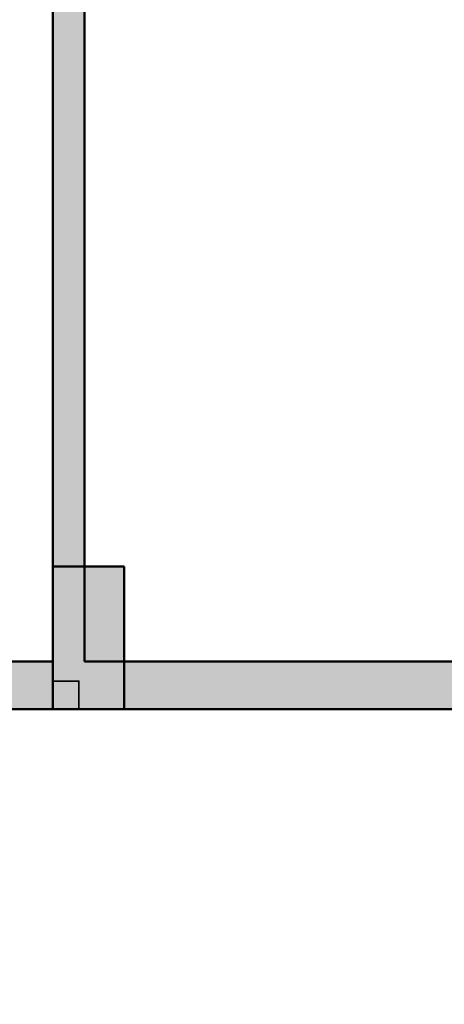
# Model space of a CAD drawing. Units: inches. Extents: x -7 to 1228, y -146 to 1091.
# Tile 58 of 88: x 376 to 429, y 531 to 655. Entities that reach past the tile are written whole.
import ezdxf

# ---------------------------------------------------------------- set-up
doc = ezdxf.new("R2010")
doc.units = ezdxf.units.IN
for name, color, linetype, lineweight in [('A-COLS', 6, 'Continuous', 35), ('A-WALL', 7, 'Continuous', 50), ('A-WALL-PATT', 251, 'Continuous', 13)]:
    doc.layers.add(name, color=color, linetype=linetype, lineweight=lineweight)

msp = doc.modelspace()

# ---------------------------------------------------------------- hatches: boundary and pattern name
at = {"layer": 'A-COLS'}
h = msp.add_hatch(color=256, dxfattribs=at)
h.dxf.hatch_style = 1
h.paths.add_polyline_path([(389, 586), (380, 586), (380, 571.55), (383.29, 571.55), (383.29, 568), (389, 568)])
h = msp.add_hatch(color=256, dxfattribs=at)
h.dxf.hatch_style = 1
h.paths.add_polyline_path([(383.29, 571.55), (380, 571.55), (380, 568), (383.29, 568)])
at = {"layer": 'A-WALL-PATT'}
h = msp.add_hatch(color=256, dxfattribs=at)
h.dxf.hatch_style = 1
h.paths.add_polyline_path([(69, 568), (60, 568), (60, 493), (63.29, 493), (69, 493)])
h.paths.add_polyline_path([(69, 662.41), (60, 662.41), (60, 586), (69, 586)], flags=17)
h.paths.add_polyline_path([(69, 723), (184, 723), (184, 734), (179, 734), (179, 728), (69, 728), (69, 741.62), (60, 741.62), (60, 698.41), (69, 698.41)], flags=17)
h.paths.add_polyline_path([(69, 782), (231, 782), (231, 728), (231, 723), (231, 586), (236, 586), (236, 787), (69, 787), (69, 800.13), (60, 800.13), (60, 765.62), (69, 765.62)])
h.paths.add_polyline_path([(184, 842), (189, 842), (189, 848), (173, 848), (173, 842), (179, 842), (179, 787), (184, 787)])
h.paths.add_polyline_path([(118.22, 69), (69, 69), (69, 60), (118.22, 60)])
h.paths.add_polyline_path([(227, 69), (154.22, 69), (154.22, 60), (227, 60)])
h.paths.add_polyline_path([(236, 60), (232.71, 60), (227, 60), (227, 36), (236, 36)])
h.paths.add_polyline_path([(389, 60), (380, 60), (380, 36), (389, 36)])
h.paths.add_polyline_path([(384, 181), (380, 181), (380, 115), (380, 78), (384, 78)])
h.paths.add_polyline_path([(380, 115), (334.55, 115), (334.55, 109), (380, 109)])
h.paths.add_polyline_path([(274.55, 115), (236, 115), (236, 201), (232.71, 201), (231, 201), (231, 78), (236, 78), (236, 109), (274.55, 109)])
h.paths.add_polyline_path([(69, 123), (60, 123), (60, 78), (69, 78)])
h.paths.add_polyline_path([(69, 201), (60, 201), (60, 159), (69, 159)])
h.paths.add_polyline_path([(143, 219), (69, 219), (69, 213), (143, 213)], flags=17)
h.paths.add_polyline_path([(189, 219), (184, 219), (184, 274), (231, 274), (231, 219), (236, 219), (236, 279), (184, 279), (184, 297), (179, 297), (179, 279), (69, 279), (69, 290.91), (60, 290.91), (60, 262.18), (69, 262.18), (69, 274), (179, 274), (179, 219), (173, 219), (173, 213), (189, 213)])
h.paths.add_polyline_path([(69, 238.18), (60, 238.18), (60, 219), (69, 219)], flags=17)
h.paths.add_polyline_path([(69, 333), (60, 333), (60, 314.91), (69, 314.91), (69, 316.96)])
h.paths.add_polyline_path([(190, 338), (184, 338), (69, 338), (69, 333), (179, 333), (179, 327), (184, 327), (184, 333.02), (190, 333.05)])
h.paths.add_polyline_path([(69, 386.81), (60, 386.81), (60, 351), (69, 351)])
h.paths.add_polyline_path([(69, 475), (60, 475), (60, 422.81), (69, 422.81)])
h.paths.add_polyline_path([(236, 475), (231, 475), (231, 351.24), (236, 351.24)])
h.paths.add_polyline_path([(384, 475), (380, 475), (380, 362), (384, 362)])
h.paths.add_polyline_path([(547, 307), (439, 307), (439, 356), (445, 356), (445, 362), (433, 362), (433, 307), (380, 307), (380, 244), (380, 241), (384, 241), (384, 301), (433, 301), (433, 277), (439, 277), (439, 301), (547, 301)])
h.paths.add_polyline_path([(547, 241), (439, 241), (439, 247), (433, 247), (433, 235), (547, 235)])
h.paths.add_polyline_path([(450, 69), (440.29, 69), (424.89, 69), (389, 69), (389, 60), (450, 60)])
h.paths.add_polyline_path([(547, 69), (486, 69), (486, 60), (547, 60)])
h.paths.add_polyline_path([(556, 148.27), (547, 148.27), (547, 78), (556, 78)])
h.paths.add_polyline_path([(556, 223), (547, 223), (547, 195), (547, 184.27), (556, 184.27)])
h.paths.add_polyline_path([(556, 311.19), (547, 311.19), (547, 273.08), (556, 273.08)])
h.paths.add_polyline_path([(556, 344), (552.71, 344), (547, 344), (547, 335.19), (556, 335.19)])
h.paths.add_polyline_path([(556, 249.08), (547, 249.08), (547, 241), (556, 241)])
h.paths.add_polyline_path([(547, 362), (475, 362), (475, 356), (547, 356)], flags=0)
h.paths.add_polyline_path([(556, 399.62), (547, 399.62), (547, 362), (556, 362)])
h.paths.add_polyline_path([(556, 475), (547, 475), (547, 435.62), (556, 435.62)])
h.paths.add_polyline_path([(547, 493), (389, 493), (389, 487), (547, 487)])
h.paths.add_polyline_path([(380, 493), (278, 493), (278, 487), (380, 487)])
h.paths.add_polyline_path([(227, 493), (69, 493), (69, 487), (227, 487)])
h.paths.add_polyline_path([(643, 122.44), (634, 122.44), (634, 78), (643, 78)])
h.paths.add_polyline_path([(702.5, 69), (692.79, 69), (677.39, 69), (643, 69), (643, 60), (702.5, 60)])
h.paths.add_polyline_path([(798, 69), (738.5, 69), (738.5, 60), (798, 60)])
h.paths.add_polyline_path([(807, 60), (803.71, 60), (798, 60), (798, 36), (807, 36)])
h.paths.add_polyline_path([(807, 109), (846.75, 109), (846.75, 115), (807, 115), (807, 159), (802, 159), (802, 78), (807, 78)])
h.paths.add_polyline_path([(807, 201), (802, 201), (802, 195), (807, 195)])
h.paths.add_polyline_path([(643, 201), (634, 201), (634, 158.44), (643, 158.44)])
h.paths.add_polyline_path([(756, 225), (751, 225), (751, 219), (643, 219), (643, 213), (756, 213)])
h.paths.add_polyline_path([(643, 240.85), (634, 240.85), (634, 219), (643, 219)])
h.paths.add_polyline_path([(643, 274), (643, 288.63), (634, 288.63), (634, 264.85), (643, 264.85)])
h.paths.add_polyline_path([(802, 279), (756, 279), (756, 297), (751, 297), (751, 279), (643, 279), (643, 274), (751, 274), (751, 255), (756, 255), (756, 274), (802, 274)])
h.paths.add_polyline_path([(807, 333), (803.71, 333), (802, 333), (802, 279), (802, 274), (802, 219), (807, 219)])
h.paths.add_polyline_path([(956, 182), (951, 182), (951, 115), (906.75, 115), (906.75, 109), (951, 109), (951, 78), (956, 78)])
h.paths.add_polyline_path([(960, 60), (951, 60), (951, 36), (960, 36)])
h.paths.add_polyline_path([(1021, 69), (1005.78, 69), (960, 69), (960, 60), (1021, 60)])
h.paths.add_polyline_path([(956, 224), (951, 224), (951, 218), (956, 218)])
h.paths.add_polyline_path([(956, 302), (1004, 302), (1004, 278), (1010, 278), (1010, 302), (1118, 302), (1118, 290.81), (1127, 290.81), (1127, 326.97), (1118, 326.97), (1118, 320.97), (1118, 307), (1010, 307), (1010, 356), (1016, 356), (1016, 362), (1004, 362), (1004, 307), (951, 307), (951, 244), (951, 242), (954.29, 242), (956, 242)])
h.paths.add_polyline_path([(643, 333), (634, 333), (634, 312.63), (643, 312.63), (643, 316.96)])
h.paths.add_polyline_path([(756, 338), (643, 338), (643, 333), (751, 333), (751, 327), (756, 327)])
h.paths.add_polyline_path([(643, 388), (634, 388), (634, 351), (643, 351)])
h.paths.add_polyline_path([(807, 357), (802, 357), (802, 351), (807, 351)])
h.paths.add_polyline_path([(807, 475), (802, 475), (802, 393), (807, 393)])
h.paths.add_polyline_path([(643, 475), (634, 475), (634, 424), (643, 424)])
h.paths.add_polyline_path([(798, 493), (643, 493), (643, 487), (798, 487)])
h.paths.add_polyline_path([(634, 493), (556, 493), (556, 487), (634, 487)])
h.paths.add_polyline_path([(813, 493), (807, 493), (807, 487), (813, 487)])
h.paths.add_polyline_path([(951, 493), (849, 493), (849, 487), (951, 487)])
h.paths.add_polyline_path([(956, 484), (951, 484), (951, 374), (956, 374)])
h.paths.add_polyline_path([(1109, 493), (969, 493), (969, 487), (1109, 487)])
h.paths.add_polyline_path([(1127, 484), (1118, 484), (1118, 450.64), (1127, 450.64)])
h.paths.add_polyline_path([(1127, 414.64), (1118, 414.64), (1118, 365), (1127, 365)])
h.paths.add_polyline_path([(1109, 362), (1046, 362), (1046, 356), (1109, 356)], flags=17)
h.paths.add_polyline_path([(1127, 356), (1123.45, 356), (1118, 356), (1118, 350.97), (1127, 350.97)], flags=0)
h.paths.add_polyline_path([(1127, 266.81), (1118, 266.81), (1118, 262.36), (1118, 242), (1127, 242)], flags=17)
h.paths.add_polyline_path([(1118, 242), (1010, 242), (1010, 248), (1004, 248), (1004, 237), (1118, 237)])
h.paths.add_polyline_path([(1127, 224), (1118, 224), (1118, 170), (1127, 170)])
h.paths.add_polyline_path([(1127, 134), (1118, 134), (1118, 78), (1127, 78)])
h.paths.add_polyline_path([(1118, 69), (1057, 69), (1057, 60), (1118, 60)])
h.paths.add_polyline_path([(227, 571.55), (227, 574), (69, 574), (69, 568), (227, 568)])
h.paths.add_polyline_path([(380, 571.55), (380, 574), (278, 574), (278, 568), (380, 568)])
h.paths.add_polyline_path([(242, 574), (236, 574), (236, 568), (242, 568)])
h.paths.add_polyline_path([(547, 571.55), (547, 574), (389, 574), (389, 568), (547, 568)])
h.paths.add_polyline_path([(384, 733), (380, 733), (380, 586), (384, 586)])
h.paths.add_polyline_path([(556, 646), (634, 646), (634, 655), (547, 655), (547, 586), (556, 586)])
h.paths.add_polyline_path([(634, 574), (556, 574), (556, 568), (634, 568)])
h.paths.add_polyline_path([(643, 655), (634, 655), (634, 586), (643, 586)])
h.paths.add_polyline_path([(798, 574), (643, 574), (643, 568), (798, 568)])
h.paths.add_polyline_path([(643, 663.85), (634, 663.85), (634, 655), (643, 655)])
h.paths.add_polyline_path([(556, 676.97), (547, 676.97), (547, 655), (556, 655)])
h.paths.add_polyline_path([(556, 733), (547, 733), (547, 712.97), (556, 712.97)])
h.paths.add_polyline_path([(643, 710), (634, 710), (634, 699.85), (643, 699.85)])
h.paths.add_polyline_path([(807, 668), (802, 668), (802, 586), (807, 586)])
h.paths.add_polyline_path([(951, 574), (849, 574), (849, 568), (951, 568)])
h.paths.add_polyline_path([(956, 691), (951, 691), (951, 577), (956, 577)])
h.paths.add_polyline_path([(1109, 574), (969, 574), (969, 568), (1109, 568)])
h.paths.add_polyline_path([(1127, 643.4), (1118, 643.4), (1118, 577), (1127, 577)])
h.paths.add_polyline_path([(1127, 568), (1123.45, 568), (1118, 568), (1118, 493), (1127, 493)])
h.paths.add_polyline_path([(1127, 733), (1118, 733), (1118, 679.4), (1127, 679.4)])
h.paths.add_polyline_path([(1127, 777.35), (1118, 777.35), (1118, 770.04), (1118, 751), (1127, 751)], flags=17)
h.paths.add_polyline_path([(1118, 751), (1010, 751), (1010, 757), (1004, 757), (1004, 745), (1118, 745)])
h.paths.add_polyline_path([(956, 811), (1004, 811), (1004, 787), (1010, 787), (1010, 811), (1017.87, 811), (1017.87, 811.63, -0.414214), (1018.25, 812), (1031.98, 812, -0.414214), (1032.35, 811.63), (1032.35, 811), (1118, 811), (1118, 801.35), (1127, 801.35), (1127, 834.69), (1118, 834.69), (1118, 830.24), (1118, 817), (1010, 817), (1010, 866), (1016, 866), (1016, 872), (1004, 872), (1004, 817), (956, 817), (956, 866), (951, 866), (951, 751), (954.29, 751), (956, 751)])
h.paths.add_polyline_path([(1118, 872), (1046, 872), (1046, 866), (1118, 866)], flags=17)
h.paths.add_polyline_path([(1127, 924.71), (1118, 924.71), (1118, 884), (1127, 884)])
h.paths.add_polyline_path([(1127, 866), (1123.71, 866), (1118, 866), (1118, 858.69), (1127, 858.69)], flags=17)
h.paths.add_polyline_path([(956, 983), (951, 983), (951, 952), (807, 952), (807, 983), (802, 983), (802, 902), (807, 902), (807, 946), (951, 946), (951, 884), (956, 884)])
h.paths.add_polyline_path([(807, 842), (802, 842), (802, 787), (756, 787), (756, 806), (751, 806), (751, 787), (643, 787), (643, 782), (751, 782), (751, 764), (756, 764), (756, 782), (802, 782), (802, 728), (807, 728)])
h.paths.add_polyline_path([(756, 848), (643, 848), (643, 842), (751, 842), (751, 836), (756, 836)])
h.paths.add_polyline_path([(756, 734), (751, 734), (751, 728), (643, 728), (643, 723), (756, 723)])
h.paths.add_polyline_path([(643, 749.79), (634, 749.79), (634, 728), (637.29, 728), (643, 728)])
h.paths.add_polyline_path([(643, 805.41), (634, 805.41), (634, 773.79), (643, 773.79)])
h.paths.add_polyline_path([(643, 896.66), (634, 896.66), (634, 860), (637.29, 860), (643, 860)])
h.paths.add_polyline_path([(643, 842), (634, 842), (634, 829.41), (643, 829.41)])
h.paths.add_polyline_path([(643, 983), (634, 983), (634, 932.66), (643, 932.66)])
h.paths.add_polyline_path([(1127, 983), (1118, 983), (1118, 960.71), (1127, 960.71)])
h.paths.add_polyline_path([(1118, 1001), (1077.53, 1001), (1077.53, 992), (1118, 992)])
h.paths.add_polyline_path([(1041.53, 1001), (960, 1001), (960, 992), (1041.53, 992)])
h.paths.add_polyline_path([(960, 1025), (951, 1025), (951, 1001), (954.29, 1001), (960, 1001)])
h.paths.add_polyline_path([(807, 1025), (798, 1025), (798, 1001), (807, 1001)])
h.paths.add_polyline_path([(798, 1001), (738.5, 1001), (738.5, 992), (798, 992)])
h.paths.add_polyline_path([(702.5, 1001), (643, 1001), (643, 992), (702.5, 992)])
h.paths.add_polyline_path([(547, 1001), (499.11, 1001), (499.11, 992), (547, 992)])
h.paths.add_polyline_path([(463.11, 1001), (389, 1001), (389, 992), (463.11, 992)])
h.paths.add_polyline_path([(389, 1025), (380, 1025), (380, 1022), (380, 1001), (383.29, 1001), (389, 1001)])
h.paths.add_polyline_path([(236, 1025), (227, 1025), (227, 1001), (236, 1001)])
h.paths.add_polyline_path([(236, 983), (231, 983), (231, 860), (236, 860)])
h.paths.add_polyline_path([(274.55, 952), (236, 952), (236, 946), (274.55, 946)])
h.paths.add_polyline_path([(380, 952), (334.55, 952), (334.55, 946), (380, 946)])
h.paths.add_polyline_path([(384, 983), (380, 983), (380, 884), (383.29, 884), (384, 884)])
h.paths.add_polyline_path([(227, 1001), (155.01, 1001), (155.01, 992), (162.87, 992), (227, 992)])
h.paths.add_polyline_path([(119.01, 1001), (69, 1001), (69, 992), (119.01, 992)])
h.paths.add_polyline_path([(69, 983), (60, 983), (60, 922.99), (69, 922.99)])
h.paths.add_polyline_path([(69, 886.99), (60, 886.99), (60, 860), (63.29, 860), (69, 860)])
h.paths.add_polyline_path([(143, 848), (69, 848), (69, 842), (143, 842)])

# ---------------------------------------------------------------- linework, layer by layer
at = {"layer": 'A-COLS'}
msp.add_lwpolyline([(380, 568), (383.29, 568), (383.29, 571.55), (380, 571.55)], close=True, dxfattribs=at)
at = {"layer": 'A-WALL'}
for p, q in [((380, 817), (380, 574)), ((384, 811), (384, 574)), ((389, 586), (380, 586)), ((380, 586), (380, 568)), ((389, 568), (389, 586)), ((380, 574), (278, 574)), ((547, 574), (384, 574)), ((380, 568), (278, 568)), ((380, 568), (389, 568)), ((547, 568), (384, 568))]:
    msp.add_line(p, q, dxfattribs=at)

doc.saveas('drawing.dxf')
